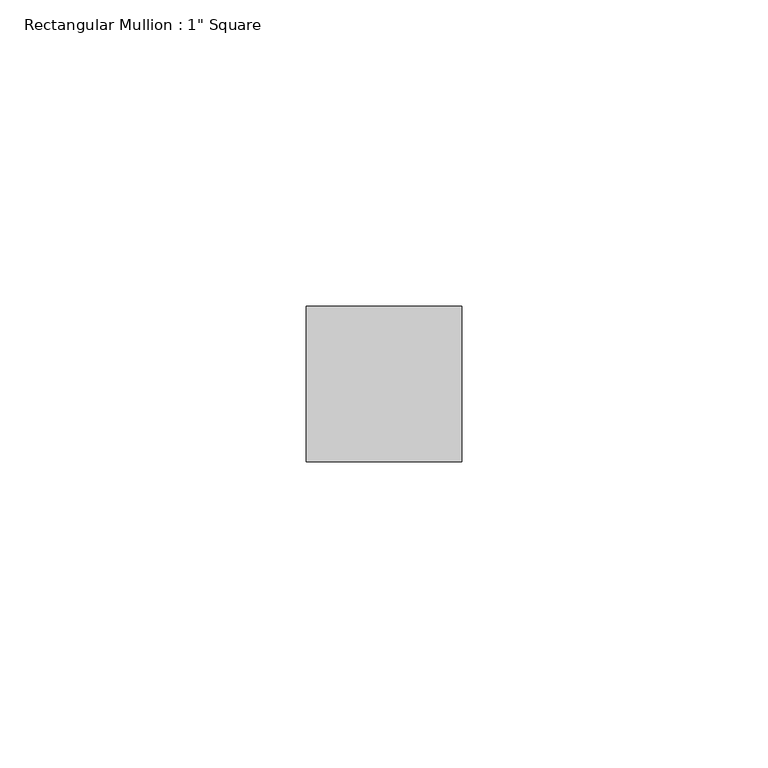
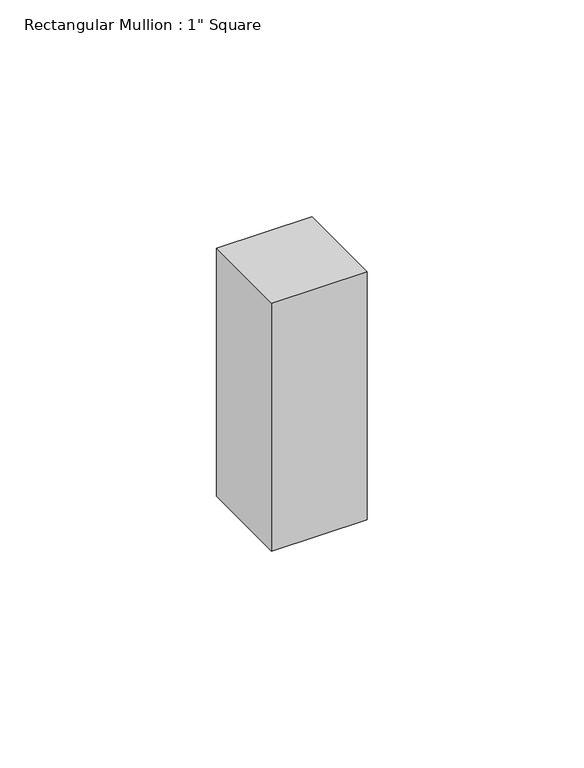
"""IFC4 building model written with IfcOpenShell, lengths in millimetres: member geometry."""

from ifc_helpers import new_model, si_unit, frame, origin, place, context, project, spatial, polyline, outline, extrude, source, transform, mapped, element, save


def member_b36ee676(model_context):
    return source(origin(), model_context, "Body", "SweptSolid", [
        extrude(outline(polyline([(0.0, 12.7), (0.0, -12.7), (-25.4, -12.7), (-25.4, 12.7), (0.0, 12.7)])), frame((0.0, 0.0, -69.85), z_axis=(0.0, 0.0, 1.0), x_axis=(1.0, 0.0, 0.0)), (0.0, 0.0, 1.0), 69.85),
    ])


if __name__ == "__main__":
    model = new_model("IFC4")
    model_context = context("Model", 3, world=origin())
    ifc_project = project(units=[si_unit("LENGTHUNIT", "METRE", prefix="MILLI")], contexts=[model_context])
    site = spatial("IfcSite", under=ifc_project)
    building = spatial("IfcBuilding", under=site)
    placement = place(None, origin())
    member_shape = member_b36ee676(model_context)
    element("IfcMember", 1, ObjectType="Rectangular Mullion : 1\" Square", at=placement, inside=building, context=model_context, shape_type="MappedRepresentation", body=[
        mapped(member_shape, transform((0.0, 0.0, 0.0), x_axis=(1.0, 0.0, 0.0), y_axis=(0.0, 1.0, 0.0), z_axis=(0.0, 0.0, 1.0))),
    ])
    save(model, "model.ifc")

# Revit data of these elements
# Type "Rectangular Mullion : 1\" Square"
#   built-in parameter 1007304 = 0.0833333 (stored number, unit not read)
#   built-in parameter 1007301 = 0.0416667 (stored number, unit not read)
#   built-in parameter 1007300 = 0.0416667 (stored number, unit not read)
# Element 1 (IfcMember, "Rectangular Mullion : 1\" Square")
#   Materials on its faces: "black"
# Materials
#   "black": class "Generic", colour RGB 120 120 120, transparency 0, Cost = 0
